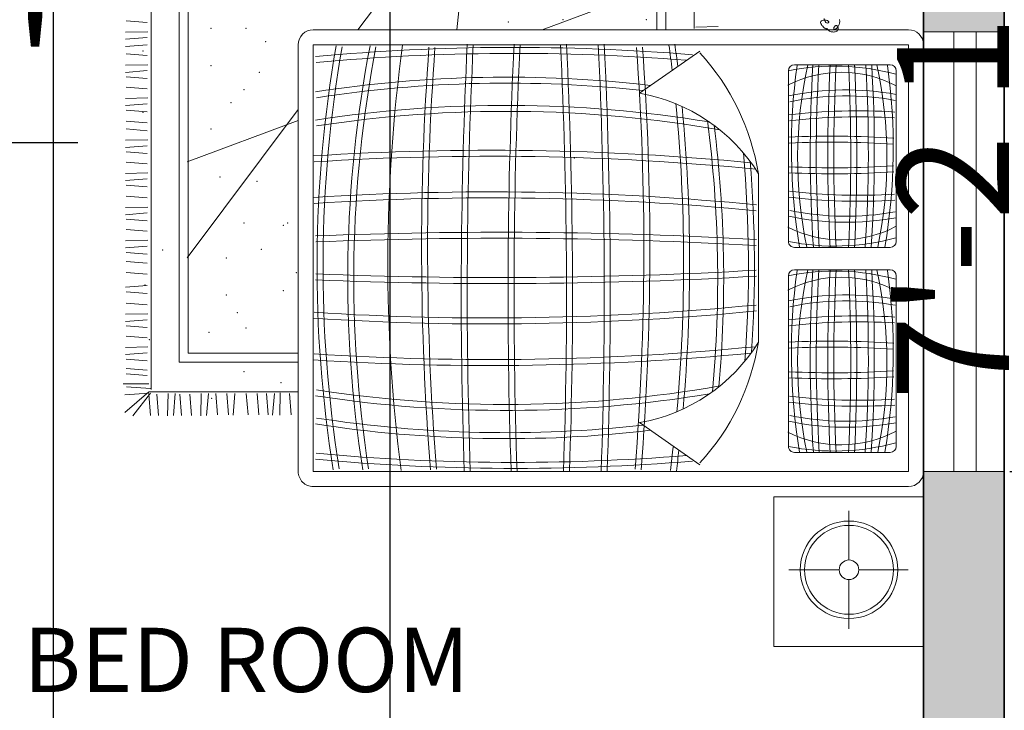
# Model space of a CAD drawing. Units: inches. Extents: x 1763 to 2368, y 1500 to 2097.
# Tile 14 of 24: x 2079 to 2189, y 1720 to 1797. Entities that reach past the tile are written whole.
import ezdxf

# ---------------------------------------------------------------- set-up
doc = ezdxf.new("R2010")
doc.units = ezdxf.units.IN
for name, color, linetype, lineweight in [('A-ANNO-DIMS', 2, 'Continuous', 18), ('A-AREA-IDEN', 7, 'Continuous', 18), ('A-FURN', 8, 'Continuous', 18), ('A-WALL', 7, 'Continuous', 35), ('A-WALL-PATT', 7, 'Continuous', 13), ('windows', 1, 'Continuous', 18)]:
    doc.layers.add(name, color=color, linetype=linetype, lineweight=lineweight)
doc.styles.get("Standard").update_dxf_attribs({"font": 'arial.ttf'})
doc.dimstyles.new('ISO-25', dxfattribs={"dimtxt": 12.5, "dimasz": 2.5, "dimexe": 1.25, "dimexo": 0.625, "dimtad": 1, "dimdec": 0, "dimlunit": 4, "dimtxsty": 'Standard', "dimblk": 'ARCHTICK', "dimcen": 2.5, "dimclrd": 3, "dimclrt": 4, "dimadec": 0, "dimazin": 0, "dimtfac": 1, "dimtdec": 0, "dimtmove": 0, "dimatfit": 3, "dimfxl": 1, "dimarcsym": 0})

# ---------------------------------------------------------------- blocks, each defined once
blk = doc.blocks.new('A$C77DF40FE')
for p, q in [((0.5839, 2.6714), (2.0097, 2.6714)), ((2.0936, 2.1723), (2.0936, 2.6723)), ((2.0936, 2.6723), (2.5936, 2.6723)), ((2.5936, 2.6723), (2.5936, 2.1723)), ((0.5339, 0.6344), (0.5339, 2.6214)), ((0.5839, 2.6214), (2.0097, 2.6214)), ((0.5839, 0.6344), (0.5839, 2.6214)), ((2.0097, 2.6214), (2.0097, 0.6344)), ((2.0597, 2.6214), (2.0597, 0.6344)), ((2.3379, 2.4554), (2.3379, 2.6199)), ((1.2408, 2.5803), (0.6708, 2.5803)), ((1.9255, 2.5803), (1.3555, 2.5803)), ((0.6508, 2.5603), (0.6508, 2.2403)), ((1.2608, 2.2403), (1.2608, 2.5603)), ((1.3355, 2.5603), (1.3355, 2.2403)), ((1.9455, 2.2403), (1.9455, 2.5603)), ((2.3051, 2.4226), (2.1406, 2.4226)), ((2.5352, 2.4226), (2.3707, 2.4226)), ((0.506, 2.3917), (0.5, 2.3914)), ((0.5117, 2.391), (0.506, 2.3917)), ((0.5168, 2.3897), (0.5117, 2.391)), ((0.5212, 2.3878), (0.5168, 2.3897)), ((0.5205, 2.3816), (0.5202, 2.3804)), ((0.5202, 2.3804), (0.5202, 2.379)), ((0.5202, 2.379), (0.5206, 2.3777)), ((0.521, 2.3828), (0.5205, 2.3816)), ((0.5206, 2.3777), (0.5213, 2.3764)), ((0.5219, 2.3839), (0.521, 2.3828)), ((0.5248, 2.3858), (0.5212, 2.3878)), ((0.5213, 2.3764), (0.5224, 2.3752)), ((0.523, 2.3849), (0.5219, 2.3839)), ((0.5224, 2.3752), (0.5237, 2.374)), ((0.5244, 2.3856), (0.523, 2.3849)), ((0.5237, 2.374), (0.5252, 2.3731)), ((0.5261, 2.3861), (0.5244, 2.3856)), ((0.5277, 2.3836), (0.5248, 2.3858)), ((0.5252, 2.3731), (0.5268, 2.3723)), ((0.5279, 2.3864), (0.5261, 2.3861)), ((0.5268, 2.3723), (0.5283, 2.3719)), ((0.5298, 2.3813), (0.5277, 2.3836)), ((0.5298, 2.3864), (0.5279, 2.3864)), ((0.5283, 2.3719), (0.5297, 2.3717)), ((0.5297, 2.3717), (0.531, 2.372)), ((0.5318, 2.3861), (0.5298, 2.3864)), ((0.5313, 2.3792), (0.5298, 2.3813)), ((0.531, 2.372), (0.5319, 2.3726)), ((0.5322, 2.3771), (0.5313, 2.3792)), ((0.5338, 2.3855), (0.5318, 2.3861)), ((0.5319, 2.3726), (0.5325, 2.3738)), ((0.5326, 2.3753), (0.5322, 2.3771)), ((0.5325, 2.3738), (0.5326, 2.3753)), ((0.5356, 2.3846), (0.5338, 2.3855)), ((0.5373, 2.3832), (0.5356, 2.3846)), ((0.5387, 2.3815), (0.5373, 2.3832)), ((0.5399, 2.3794), (0.5387, 2.3815)), ((0.5407, 2.377), (0.5399, 2.3794)), ((0.5412, 2.3743), (0.5407, 2.377)), ((0.5409, 2.3657), (0.5413, 2.3686)), ((0.5414, 2.3715), (0.5412, 2.3743)), ((0.5413, 2.3686), (0.5414, 2.3715)), ((2.3379, 2.2215), (2.3379, 2.3898)), ((0.4961, 2.3402), (0.5023, 2.3413)), ((0.502, 2.3463), (0.5017, 2.3431)), ((0.5017, 2.3431), (0.5018, 2.3398)), ((0.5018, 2.3398), (0.5023, 2.3365)), ((0.5026, 2.3491), (0.502, 2.3463)), ((0.5023, 2.3413), (0.5067, 2.3431)), ((0.5023, 2.3365), (0.5031, 2.3334)), ((0.5035, 2.3514), (0.5026, 2.3491)), ((0.5031, 2.3334), (0.5043, 2.3309)), ((0.5047, 2.3531), (0.5035, 2.3514)), ((0.5059, 2.3542), (0.5047, 2.3531)), ((0.5073, 2.3548), (0.5059, 2.3542)), ((0.5067, 2.3431), (0.5095, 2.3452)), ((0.5086, 2.3549), (0.5073, 2.3548)), ((0.5097, 2.3544), (0.5086, 2.3549)), ((0.5095, 2.3452), (0.511, 2.3475)), ((0.5107, 2.3534), (0.5097, 2.3544)), ((0.5113, 2.3518), (0.5107, 2.3534)), ((0.511, 2.3475), (0.5115, 2.3498)), ((0.5115, 2.3498), (0.5113, 2.3518)), ((0.5193, 2.3325), (0.5222, 2.3349)), ((0.5222, 2.3349), (0.5249, 2.3374)), ((0.5249, 2.3374), (0.5271, 2.3398)), ((0.5271, 2.3398), (0.5288, 2.3419)), ((0.5288, 2.3419), (0.5299, 2.3436)), ((0.5299, 2.3436), (0.5305, 2.3449)), ((0.53, 2.3482), (0.5302, 2.3488)), ((0.5301, 2.3477), (0.53, 2.3482)), ((0.5303, 2.3472), (0.5301, 2.3477)), ((0.5302, 2.3488), (0.5308, 2.3495)), ((0.5306, 2.3466), (0.5303, 2.3472)), ((0.5305, 2.3449), (0.5307, 2.3459)), ((0.5307, 2.3459), (0.5306, 2.3466)), ((0.5308, 2.3495), (0.5317, 2.3504)), ((0.5317, 2.3504), (0.5329, 2.3515)), ((0.5329, 2.3515), (0.5342, 2.3528)), ((0.5342, 2.3528), (0.5356, 2.3543)), ((0.5356, 2.3543), (0.537, 2.3561)), ((0.537, 2.3561), (0.5383, 2.3581)), ((0.5383, 2.3581), (0.5394, 2.3604)), ((0.5394, 2.3604), (0.5403, 2.3629)), ((0.5403, 2.3629), (0.5409, 2.3657)), ((0.5043, 2.3309), (0.506, 2.329)), ((0.506, 2.329), (0.5081, 2.328)), ((0.5081, 2.328), (0.5106, 2.328)), ((0.5106, 2.328), (0.5134, 2.3288)), ((0.5134, 2.3288), (0.5163, 2.3304)), ((0.5163, 2.3304), (0.5193, 2.3325)), ((0.6708, 2.2203), (1.2408, 2.2203)), ((1.3555, 2.2203), (1.9255, 2.2203)), ((2.5936, 2.1723), (2.0936, 2.1723)), ((1.5773, 2.1205), (1.0147, 2.1205)), ((0.5249, 1.9118), (0.5233, 1.9865)), ((0.6051, 1.925), (0.7457, 1.7234)), ((1.9869, 1.925), (1.8463, 1.7234)), ((0.5301, 1.9057), (0.3112, 1.9057)), ((0.5339, 1.8116), (0.3112, 1.8116)), ((0.5339, 1.7816), (0.3112, 1.7816)), ((0.3909, 1.7821), (0.5339, 1.398)), ((0.5339, 1.1132), (0.2152, 1.1479)), ((0.5339, 0.7837), (0.2152, 1.0221)), ((2.0097, 0.6344), (0.5839, 0.6344)), ((2.0097, 0.5844), (0.5839, 0.5844)), ((1.2963, 0.2134), (0.8003, 0.5844)), ((0.8369, 0.5844), (0.975, 0.2134)), ((1.6139, 0.217), (1.6139, 0.5844)), ((1.6439, 0.187), (1.6439, 0.5844)), ((1.7439, 0.087), (1.7439, 0.5844)), ((1.8197, 0.5605), (1.7489, 0.5548)), ((1.8218, 0.5229), (1.7471, 0.5245)), ((1.8218, 0.499), (1.7487, 0.5048)), ((1.8197, 0.4839), (1.7489, 0.4783)), ((1.8197, 0.453), (1.7489, 0.4474)), ((1.8197, 0.4168), (1.7489, 0.4111)), ((1.8218, 0.3671), (1.7487, 0.3728)), ((1.8197, 0.352), (1.7489, 0.3463)), ((1.8197, 0.3146), (1.7489, 0.3089)), ((1.7492, 0.2844), (1.8223, 0.2787)), ((1.7492, 0.2606), (1.824, 0.2589)), ((0.3112, 0.217), (1.6139, 0.217)), ((1.7513, 0.223), (1.8221, 0.2286)), ((0.3112, 0.187), (1.6439, 0.187)), ((1.7492, 0.1737), (1.8223, 0.1679)), ((1.7513, 0.1888), (1.8221, 0.1944)), ((1.7492, 0.1499), (1.824, 0.1482)), ((1.7513, 0.1122), (1.8221, 0.1179)), ((0.3112, 0.0935), (1.0155, 0.0935)), ((0.5043, 0.0096), (0.51, 0.0804)), ((0.542, 0.0075), (0.5403, 0.0823)), ((0.5658, 0.0075), (0.56, 0.0806)), ((0.5896, 0.0075), (0.5838, 0.0806)), ((0.6147, 0.0096), (0.6204, 0.0804)), ((0.6523, 0.0075), (0.6507, 0.0823)), ((0.6762, 0.0075), (0.6704, 0.0806)), ((0.6912, 0.0096), (0.6969, 0.0804)), ((0.7254, 0.0096), (0.7311, 0.0804)), ((0.7631, 0.0075), (0.7614, 0.0823)), ((0.7869, 0.0075), (0.7811, 0.0806)), ((0.802, 0.0096), (0.8076, 0.0804)), ((0.8394, 0.0096), (0.8451, 0.0804)), ((0.8654, 0.0096), (0.8711, 0.0804)), ((0.9031, 0.0075), (0.9014, 0.0823)), ((0.9269, 0.0075), (0.9212, 0.0806)), ((0.942, 0.0096), (0.9477, 0.0804)), ((0.9762, 0.0096), (0.9818, 0.0804)), ((1.0138, 0.0075), (1.0122, 0.0823)), ((1.0155, 0.0935), (1.7355, 0.0935)), ((1.0376, 0.0075), (1.0319, 0.0806)), ((1.0527, 0.0096), (1.0584, 0.0804)), ((1.0901, 0.0096), (1.0958, 0.0804)), ((1.1278, 0.0075), (1.1261, 0.0823)), ((1.1516, 0.0075), (1.1459, 0.0806)), ((1.1667, 0.0096), (1.1724, 0.0804)), ((1.2009, 0.0096), (1.2065, 0.0804)), ((1.2385, 0.0075), (1.2368, 0.0823)), ((1.2623, 0.0075), (1.2566, 0.0806)), ((1.2774, 0.0096), (1.2831, 0.0804)), ((1.3083, 0.0096), (1.314, 0.0804)), ((1.3446, 0.0096), (1.3503, 0.0804)), ((1.3943, 0.0075), (1.3885, 0.0806)), ((1.4094, 0.0096), (1.415, 0.0804)), ((1.4468, 0.0096), (1.4525, 0.0804)), ((1.4844, 0.0075), (1.4828, 0.0823)), ((1.5083, 0.0075), (1.5025, 0.0806)), ((1.5233, 0.0096), (1.529, 0.0804)), ((1.5575, 0.0096), (1.5632, 0.0804)), ((1.5951, 0.0075), (1.5935, 0.0823)), ((1.619, 0.0075), (1.6132, 0.0806)), ((1.6341, 0.0096), (1.6397, 0.0804)), ((1.665, 0.0096), (1.6706, 0.0804)), ((1.6831, 0.0096), (1.6888, 0.0804)), ((1.7162, 0.0857), (1.7162, 0)), ((1.7323, 0.0911), (1.7269, 0.0107)), ((1.743, 0.0857), (1.8126, 0.0054)), ((1.7483, 0.0911), (1.8233, 0.0322)), ((1.7483, 0.0857), (1.7537, 0.0054)), ((1.7513, 0.0858), (1.8221, 0.0915))]:
    blk.add_line(p, q)
for radius in [0.1629, 0.1484, 0.0328]:
    blk.add_circle((2.3379, 2.4226), radius)
for centre, radius, start, end in [((0.5839, 2.6214), 0.05, 90, 180), ((2.0097, 2.6214), 0.05, 0, 90), ((0.6708, 2.5603), 0.02, 90, 180), ((0.9287, 0.5819), 1.9884, 80.4201, 97.9672), ((1.4247, 2.3742), 0.7696, 164.6112, 191.5679), ((1.0701, 2.3966), 0.3942, 152.5365, 206.92), ((1.6628, 2.4129), 0.928, 169.6087, 191.899), ((1.6628, 2.4129), 0.908, 169.6087, 191.899), ((2.7571, 2.4533), 1.9523, 176.3947, 186.8195), ((2.7571, 2.4533), 1.9323, 176.3947, 186.8195), ((3.9259, 2.3685), 3.0367, 176.1432, 182.775), ((3.9259, 2.3685), 3.0167, 176.1432, 182.775), ((-2.0216, 2.3685), 3.0167, 357.225, 3.8568), ((-2.0216, 2.3685), 3.0367, 357.225, 3.8568), ((-0.8455, 2.4533), 1.9323, 353.1805, 3.6053), ((-0.8455, 2.4533), 1.9523, 353.1805, 3.6053), ((0.2489, 2.4129), 0.908, 348.101, 10.3913), ((0.2489, 2.4129), 0.928, 348.101, 10.3913), ((0.8416, 2.3966), 0.3942, 333.08, 27.4635), ((0.4869, 2.3742), 0.7696, 348.4321, 15.3888), ((1.2408, 2.5603), 0.02, 0, 90), ((1.3555, 2.5603), 0.02, 90, 180), ((1.6135, 0.5819), 1.9884, 80.4201, 97.9672), ((2.1094, 2.3742), 0.7696, 164.6112, 191.5679), ((1.7548, 2.3966), 0.3942, 152.5365, 206.92), ((2.3475, 2.4129), 0.928, 169.6087, 191.899), ((2.3475, 2.4129), 0.908, 169.6087, 191.899), ((3.4419, 2.4533), 1.9523, 176.3947, 186.8195), ((3.4419, 2.4533), 1.9323, 176.3947, 186.8195), ((4.6106, 2.3685), 3.0367, 176.1432, 182.775), ((4.6106, 2.3685), 3.0167, 176.1432, 182.775), ((-1.3369, 2.3685), 3.0167, 357.225, 3.8568), ((-1.3369, 2.3685), 3.0367, 357.225, 3.8568), ((-0.1608, 2.4533), 1.9323, 353.1805, 3.6053), ((-0.1608, 2.4533), 1.9523, 353.1805, 3.6053), ((0.9336, 2.4129), 0.908, 348.101, 10.3913), ((0.9336, 2.4129), 0.928, 348.101, 10.3913), ((1.5263, 2.3966), 0.3942, 333.08, 27.4635), ((1.1716, 2.3742), 0.7696, 348.4321, 15.3888), ((1.9255, 2.5603), 0.02, 0, 90), ((0.9635, 1.1066), 1.4427, 78.1527, 102.4906), ((1.6482, 1.1066), 1.4427, 78.1527, 102.4906), ((0.9445, -2.3575), 4.8647, 86.2671, 93.4563), ((1.6292, -2.3575), 4.8647, 86.2671, 93.4563), ((0.9445, -2.3575), 4.8447, 86.2671, 93.4563), ((1.6292, -2.3575), 4.8447, 86.2671, 93.4563), ((0.9561, -3.928), 6.3765, 87.24779, 92.75221), ((1.6408, -3.928), 6.3765, 87.24779, 92.75221), ((0.9561, -3.928), 6.3565, 87.24779, 92.75221), ((1.6408, -3.928), 6.3565, 87.24779, 92.75221), ((0.9561, 8.7285), 6.3565, 267.24779, 272.75221), ((1.6408, 8.7285), 6.3565, 267.24779, 272.75221), ((0.9561, 8.7285), 6.3765, 267.24779, 272.75221), ((1.6408, 8.7285), 6.3765, 267.24779, 272.75221), ((0.9445, 7.158), 4.8647, 266.5437, 273.7329), ((0.9445, 7.158), 4.8447, 266.5437, 273.7329), ((1.6292, 7.158), 4.8647, 266.5437, 273.7329), ((1.6292, 7.158), 4.8447, 266.5437, 273.7329), ((0.9635, 3.6939), 1.4427, 257.5094, 281.8473), ((1.6482, 3.6939), 1.4427, 257.5094, 281.8473), ((0.6708, 2.2403), 0.02, 180, 270), ((0.9287, 4.2186), 1.9884, 262.0328, 279.5799), ((1.2408, 2.2403), 0.02, 270, 0), ((1.3555, 2.2403), 0.02, 180, 270), ((1.6135, 4.2186), 1.9884, 262.0328, 279.5799), ((1.9255, 2.2403), 0.02, 270, 0), ((1.1396, 1.3485), 0.782, 99.1908, 132.5116), ((1.3217, 1.6229), 0.5847, 121.6676, 170.1065), ((10.1174, 1.2237), 9.161, 174.43278, 183.67204), ((1.3248, -2.1722), 4.2793, 86.1532, 94.7091), ((10.2564, 1.2237), 9.181, 174.43278, 183.67204), ((10.2564, 1.2237), 9.161, 174.43278, 183.67204), ((16.3019, 1.253), 15.0916, 176.72768, 182.32074), ((16.3019, 1.253), 15.0716, 176.72768, 182.32074), ((-13.7099, 1.253), 15.0716, 357.67926, 3.27232), ((-13.7099, 1.253), 15.0916, 357.67926, 3.27232), ((-7.6644, 1.2237), 9.161, 356.32796, 5.56722), ((-7.6644, 1.2237), 9.181, 356.32796, 5.56722), ((1.2703, 1.6229), 0.5847, 9.8935, 58.3324), ((1.4523, 1.3485), 0.782, 47.4884, 80.8092), ((-7.5254, 1.2237), 9.161, 356.32796, 5.55658), ((10.1174, 1.2237), 9.181, 174.54912, 183.67204), ((1.3248, -2.1722), 4.2593, 85.7473, 95.1159), ((-7.5254, 1.2237), 9.181, 356.32796, 5.45088), ((4.947, 1.2796), 4.1406, 170.0939, 188.8179), ((1.3657, -2.1044), 4.0888, 84.7053, 97.4283), ((1.3657, -2.1044), 4.1088, 84.9619, 97.1707), ((-2.355, 1.2796), 4.1406, 351.1821, 9.9061), ((4.947, 1.2796), 4.1606, 170.6272, 188.8179), ((-2.355, 1.2796), 4.1606, 351.1821, 9.3728), ((7.8077, 1.3061), 7.2149, 175.27403, 185.28261), ((7.8077, 1.3061), 7.1949, 175.41729, 185.28261), ((1.3142, -3.5764), 5.4671, 84.8953, 95.5052), ((-5.2157, 1.3061), 7.1949, 354.71739, 4.58271), ((-5.2157, 1.3061), 7.2149, 354.71739, 4.72597), ((1.3142, -3.5764), 5.4671, 96.9078, 97.6924), ((1.3142, -3.5764), 5.4471, 84.7792, 95.6214), ((1.3142, -3.5764), 5.4671, 82.7025, 83.4474), ((1.3142, -3.5764), 5.4471, 96.796, 97.6924), ((1.3142, -3.5764), 5.4471, 82.7025, 83.5609), ((1.2659, -7.4764), 9.2344, 85.41732, 94.18368), ((4.8527, 1.2796), 4.1606, 173.3677, 188.8179), ((-2.2608, 1.2796), 4.1606, 351.1821, 6.6323), ((1.2659, -7.4764), 9.2144, 85.41732, 94.18368), ((4.8527, 1.2796), 4.1406, 173.6812, 188.8179), ((-2.2608, 1.2796), 4.1406, 351.1821, 6.3188), ((1.4138, -15.5462), 17.172, 88.01473, 92.775), ((1.4138, -15.5462), 17.152, 88.01473, 92.775), ((1.4138, -15.6721), 17.172, 88.01473, 92.775), ((1.4138, -15.6721), 17.152, 88.01473, 92.775), ((1.4138, 18.4566), 17.152, 267.225, 271.98527), ((1.4138, 18.4566), 17.172, 267.225, 271.98527), ((1.4138, 18.3004), 17.152, 267.225, 271.98527), ((1.4138, 18.3004), 17.172, 267.225, 271.98527), ((1.2659, 10.2305), 9.2344, 265.81632, 274.58268), ((1.2659, 10.2305), 9.2144, 265.81632, 274.58268), ((1.3142, 6.3306), 5.4471, 262.3076, 277.2975), ((1.3657, 4.8586), 4.1088, 259.0794, 278.9327), ((1.3657, 4.8586), 4.0888, 259.0794, 278.9327), ((1.3248, 4.9264), 4.2593, 260.0761, 279.1287), ((1.3248, 4.9264), 4.2793, 260.0761, 279.1287), ((0.5839, 0.6344), 0.05, 180, 270), ((2.0097, 0.6344), 0.05, 270, 0)]:
    blk.add_arc(centre, radius, start, end)
for p in [(0.5004, 1.7457), (0.9622, 1.5058), (0.5004, 1.4684), (0.5077, 1.286), (1.3453, 0.5782), (1.1794, 0.5491), (1.1867, 0.5345), (1.4058, 0.5345), (1.7124, 0.5272), (0.5734, 0.4761), (1.2671, 0.4615), (0.6757, 0.4542), (1.0407, 0.4469), (0.5296, 0.4104), (0.7341, 0.4032), (1.1794, 0.4032), (1.5299, 0.4104), (1.6759, 0.4032), (1.4788, 0.3813), (0.7779, 0.3594), (1.2963, 0.3448), (1.4204, 0.3448), (1.0261, 0.3229), (0.5296, 0.2937), (0.6538, 0.2937), (0.8655, 0.2937), (1.5445, 0.2864), (1.7652, 0.2958), (1.2693, 0.1315), (0.6049, 0.0659), (0.8093, 0.0659), (1.3861, 0.0732), (1.5686, 0.0878)]:
    blk.add_point(p)
blk = doc.blocks.new('_ArchTick')
at = {"color": 0, "linetype": 'ByBlock', "const_width": 0.15}
blk.add_lwpolyline([(-0.5, -0.5), (0.5, 0.5)], dxfattribs=at)
blk = doc.blocks.new('*D22')
at = {"layer": 'A-ANNO-DIMS', "color": 0, "lineweight": -2, "transparency": 16777216}
for p, q in [((2189.72, 2043.27), (2269.32, 2043.27)), ((2268.07, 2043.27), (2268.07, 1563.27)), ((2189.72, 1563.27), (2269.32, 1563.27))]:
    blk.add_line(p, q, dxfattribs=at)
at = {"layer": 'Defpoints', "color": 0, "transparency": 16777216}
for p in [(2189.09, 2043.27), (2189.09, 1563.27), (2268.07, 1563.27)]:
    blk.add_point(p, dxfattribs=at)
at = {"layer": 'A-ANNO-DIMS', "color": 0, "lineweight": -2, "transparency": 16777216, "xscale": 2.5, "yscale": 2.5, "zscale": 2.5}
for p, rotation in [((2268.07, 2043.27), 90), ((2268.07, 1563.27), 270)]:
    blk.add_blockref('_ArchTick', p, dxfattribs=dict(at, rotation=rotation))
at = {"layer": 'A-ANNO-DIMS', "color": 0, "transparency": 16777216, "insert": (2261.06, 1803.27), "char_height": 12.5, "attachment_point": 5, "rotation": 90}
blk.add_mtext("40'", dxfattribs=at)
blk = doc.blocks.new('*D24')
at = {"layer": 'A-ANNO-DIMS', "color": 0, "lineweight": -2, "transparency": 16777216}
for p, q in [((2179.32, 1949.35), (2193.33, 1949.35)), ((2179.32, 1862.76), (2193.33, 1862.76))]:
    blk.add_line(p, q, dxfattribs=at)
at = {"layer": 'A-ANNO-DIMS', "color": 3, "lineweight": -2, "transparency": 16777216}
for p, q in [((2192.08, 1949.35), (2192.08, 1862.76)), ((2192.08, 1862.76), (2192.08, 1753.79))]:
    blk.add_line(p, q, dxfattribs=at)
at = {"layer": 'Defpoints', "color": 0, "transparency": 16777216}
for p in [(2178.7, 1949.35), (2178.7, 1862.76), (2192.08, 1862.76)]:
    blk.add_point(p, dxfattribs=at)
at = {"layer": 'A-ANNO-DIMS', "color": 3, "lineweight": -2, "transparency": 16777216, "xscale": 2.5, "yscale": 2.5, "zscale": 2.5}
for p, rotation in [((2192.08, 1949.35), 90), ((2192.08, 1862.76), 270)]:
    blk.add_blockref('_ArchTick', p, dxfattribs=dict(at, rotation=rotation))
at = {"layer": 'A-ANNO-DIMS', "color": 4, "transparency": 16777216, "insert": (2184.99, 1807.02), "char_height": 12.5, "attachment_point": 5, "rotation": 90}
blk.add_mtext('7\'-2 1/2" TYP.', dxfattribs=at)
blk = doc.blocks.new('*D27')
at = {"layer": 'A-ANNO-DIMS', "color": 0, "lineweight": -2, "transparency": 16777216}
for p, q in [((1853.71, 1795.96), (1853.71, 1781.68)), ((1944.71, 1795.96), (1944.71, 1781.68))]:
    blk.add_line(p, q, dxfattribs=at)
at = {"layer": 'A-ANNO-DIMS', "color": 3, "lineweight": -2, "transparency": 16777216}
for p, q in [((1853.71, 1782.93), (1944.71, 1782.93)), ((1944.71, 1782.93), (2085.85, 1782.93))]:
    blk.add_line(p, q, dxfattribs=at)
at = {"layer": 'Defpoints', "color": 0, "transparency": 16777216}
for p in [(1853.71, 1796.58), (1944.71, 1796.58), (1944.71, 1782.93)]:
    blk.add_point(p, dxfattribs=at)
at = {"layer": 'A-ANNO-DIMS', "color": 3, "lineweight": -2, "transparency": 16777216, "xscale": 2.5, "yscale": 2.5, "zscale": 2.5, "rotation": 180}
blk.add_blockref('_ArchTick', (1853.71, 1782.93), dxfattribs=at)
at = {"layer": 'A-ANNO-DIMS', "color": 3, "lineweight": -2, "transparency": 16777216, "xscale": 2.5, "yscale": 2.5, "zscale": 2.5}
blk.add_blockref('_ArchTick', (1944.71, 1782.93), dxfattribs=at)
at = {"layer": 'A-ANNO-DIMS', "color": 4, "transparency": 16777216, "insert": (2016.53, 1790.02), "char_height": 12.5, "attachment_point": 5}
blk.add_mtext('DINING SET 7\'-7"', dxfattribs=at)
blk = doc.blocks.new('*D52')
at = {"layer": 'A-ANNO-DIMS', "color": 0, "lineweight": -2, "transparency": 16777216}
for p, q in [((2189.72, 1746.22), (2217.84, 1746.22)), ((2180.72, 1679.27), (2217.84, 1679.27))]:
    blk.add_line(p, q, dxfattribs=at)
at = {"layer": 'A-ANNO-DIMS', "color": 3, "lineweight": -2, "transparency": 16777216}
blk.add_line((2216.59, 1679.27), (2216.59, 1746.22), dxfattribs=at)
at = {"layer": 'Defpoints', "color": 0, "transparency": 16777216}
for p in [(2189.09, 1746.22), (2216.59, 1746.22), (2180.09, 1679.27)]:
    blk.add_point(p, dxfattribs=at)
at = {"layer": 'A-ANNO-DIMS', "color": 3, "lineweight": -2, "transparency": 16777216, "xscale": 2.5, "yscale": 2.5, "zscale": 2.5}
for p, rotation in [((2216.59, 1746.22), 90), ((2216.59, 1679.27), 270)]:
    blk.add_blockref('_ArchTick', p, dxfattribs=dict(at, rotation=rotation))
at = {"layer": 'A-ANNO-DIMS', "color": 4, "transparency": 16777216, "insert": (2209.61, 1712.75), "char_height": 12.5, "attachment_point": 5, "rotation": 90}
blk.add_mtext('5\'-7"', dxfattribs=at)
blk = doc.blocks.new('*D62')
at = {"layer": 'A-ANNO-DIMS', "color": 0, "lineweight": -2, "transparency": 16777216}
for p, q in [((2083.09, 1980.65), (2083.09, 1509.91)), ((2120.61, 1980.65), (2120.61, 1509.91))]:
    blk.add_line(p, q, dxfattribs=at)
at = {"layer": 'A-ANNO-DIMS', "color": 3, "lineweight": -2, "transparency": 16777216}
for p, q in [((2083.09, 1511.16), (2120.61, 1511.16)), ((2120.61, 1511.16), (2186.71, 1511.16))]:
    blk.add_line(p, q, dxfattribs=at)
at = {"layer": 'Defpoints', "color": 0, "transparency": 16777216}
for p in [(2083.09, 1981.27), (2120.61, 1981.27), (2120.61, 1511.16)]:
    blk.add_point(p, dxfattribs=at)
at = {"layer": 'A-ANNO-DIMS', "color": 3, "lineweight": -2, "transparency": 16777216, "xscale": 2.5, "yscale": 2.5, "zscale": 2.5, "rotation": 180}
blk.add_blockref('_ArchTick', (2083.09, 1511.16), dxfattribs=at)
at = {"layer": 'A-ANNO-DIMS', "color": 3, "lineweight": -2, "transparency": 16777216, "xscale": 2.5, "yscale": 2.5, "zscale": 2.5}
blk.add_blockref('_ArchTick', (2120.61, 1511.16), dxfattribs=at)
at = {"layer": 'A-ANNO-DIMS', "color": 4, "transparency": 16777216, "insert": (2154.91, 1518.25), "char_height": 12.5, "attachment_point": 5}
blk.add_mtext('3\'-1 1/2"', dxfattribs=at)
blk = doc.blocks.new('*D71')
at = {"layer": 'A-ANNO-DIMS', "color": 0, "lineweight": -2, "transparency": 16777216}
for p, q in [((2049.69, 1879.65), (2049.69, 1509.91)), ((2072.78, 1879.65), (2072.78, 1509.91))]:
    blk.add_line(p, q, dxfattribs=at)
at = {"layer": 'A-ANNO-DIMS', "color": 3, "lineweight": -2, "transparency": 16777216}
for p, q in [((2049.69, 1511.16), (2072.78, 1511.16)), ((2072.78, 1511.16), (2118.3, 1511.16))]:
    blk.add_line(p, q, dxfattribs=at)
at = {"layer": 'Defpoints', "color": 0, "transparency": 16777216}
for p in [(2049.69, 1880.27), (2072.78, 1880.27), (2072.78, 1511.16)]:
    blk.add_point(p, dxfattribs=at)
at = {"layer": 'A-ANNO-DIMS', "color": 3, "lineweight": -2, "transparency": 16777216, "xscale": 2.5, "yscale": 2.5, "zscale": 2.5, "rotation": 180}
blk.add_blockref('_ArchTick', (2049.69, 1511.16), dxfattribs=at)
at = {"layer": 'A-ANNO-DIMS', "color": 3, "lineweight": -2, "transparency": 16777216, "xscale": 2.5, "yscale": 2.5, "zscale": 2.5}
blk.add_blockref('_ArchTick', (2072.78, 1511.16), dxfattribs=at)
at = {"layer": 'A-ANNO-DIMS', "color": 4, "transparency": 16777216, "insert": (2096.79, 1518.06), "char_height": 12.5, "attachment_point": 5}
blk.add_mtext('1\'-11"', dxfattribs=at)

msp = doc.modelspace()

# ---------------------------------------------------------------- hatches: boundary and pattern name
at = {"layer": 'A-WALL-PATT'}
h = msp.add_hatch(color=256, dxfattribs=at)
h.dxf.hatch_style = 1
h.paths.add_polyline_path([(1838.09, 2034.27), (1838.09, 2043.27), (1829.09, 2043.27), (1829.09, 1953.39), (1838.09, 1953.39)])
h.paths.add_polyline_path([(1838.09, 1913.1), (1829.09, 1913.1), (1829.09, 1862.2), (1838.09, 1862.2)])
h.paths.add_polyline_path([(1838.09, 1825.59), (1829.09, 1825.59), (1829.09, 1738.64), (1838.09, 1738.64)])
h.paths.add_polyline_path([(1895.59, 1885.27), (1838.09, 1885.27), (1838.09, 1880.27), (1895.59, 1880.27)])
h.paths.add_polyline_path([(1857.39, 1784.27), (1838.09, 1784.27), (1838.09, 1779.27), (1857.39, 1779.27)])
h.paths.add_polyline_path([(1958.09, 1981.27), (1971.46, 1981.27), (1971.46, 1986.27), (1968.57, 1986.27), (1958.09, 1986.27), (1953.09, 1986.27), (1927.39, 1986.27), (1927.39, 1981.27), (1953.09, 1981.27), (1953.09, 1885.27), (1932.01, 1885.27), (1932.01, 1880.27), (1959.13, 1880.27), (1959.13, 1883.74), (1959.13, 1885.27), (1958.09, 1885.27)])
h.paths.add_polyline_path([(2018.09, 1981.27), (2031.02, 1981.27), (2031.02, 1986.27), (2018.09, 1986.27), (2013.09, 1986.27), (2001.23, 1986.27), (2001.23, 1981.27), (2013.09, 1981.27), (2013.09, 1885.27), (1982.18, 1885.27, -0.016629), (1982.23, 1883.74), (1982.23, 1880.27), (2049.69, 1880.27), (2049.69, 1883.74, -0.016629), (2049.74, 1885.27), (2018.09, 1885.27)])
h.paths.add_polyline_path([(2083.09, 1981.27), (2120.61, 1981.27), (2120.61, 1986.27), (2083.09, 1986.27), (2078.09, 1986.27), (2063.14, 1986.27), (2063.14, 1981.27), (2078.09, 1981.27), (2078.09, 1885.27), (2072.78, 1885.27), (2072.78, 1883.74), (2072.78, 1880.27), (2078.09, 1880.27), (2078.09, 1866.87), (2081.56, 1866.87, -0.016629), (2083.09, 1866.82)])
h.paths.add_polyline_path([(1871.68, 1635.27), (1838.09, 1635.27), (1838.09, 1626.27), (1871.68, 1626.27)], flags=17)
h.paths.add_polyline_path([(2100.58, 1688.27), (2060.09, 1688.27), (2060.09, 1679.27), (2100.58, 1679.27)], flags=17)
h.paths.add_polyline_path([(2180.09, 1688.27), (2148.74, 1688.27), (2148.74, 1679.27), (2180.09, 1679.27)], flags=17)
h.paths.add_polyline_path([(2189.09, 1746.22), (2180.09, 1746.22), (2180.09, 1743.42), (2180.12, 1743.42), (2180.12, 1726.72), (2180.09, 1572.27), (2034.91, 1572.27), (2034.91, 1565.6), (2034.91, 1563.27), (2189.09, 1563.27)])
h.paths.add_polyline_path([(2060.09, 1802.35, -0.016629), (2058.56, 1802.3), (2055.09, 1802.3), (2055.09, 1635.27), (2042.48, 1635.27), (2042.48, 1629.74), (2042.48, 1626.27), (2055.09, 1626.27), (2055.09, 1599.27), (2040.27, 1599.27), (2040.27, 1590.27), (2060.09, 1590.27)])
h.paths.add_polyline_path([(2019.39, 1629.74, -0.060569), (2020.06, 1635.27), (1995.09, 1635.27), (1990.09, 1635.27), (1927.07, 1635.27), (1927.07, 1626.27), (1990.09, 1626.27), (1990.09, 1590.27), (1995.09, 1590.27), (2005.2, 1590.27), (2005.2, 1599.27), (1995.09, 1599.27), (1995.09, 1626.27), (2019.39, 1626.27)])
edge = h.paths.add_edge_path()
edge.add_line((2180.09, 1837.27), (2167.2, 1837.27))
edge.add_spline(control_points=[(2167.2, 1837.27), (2167.19, 1837.27), (2167.18, 1837.27), (2167.18, 1837.27)], knot_values=[168.955493, 168.955493, 168.955493, 168.955493, 169.065871, 169.065871, 169.065871, 169.065871], degree=3, periodic=0)
edge.add_spline(control_points=[(2167.18, 1837.27), (2166.56, 1837.38), (2166.33, 1846.16), (2165.71, 1846.24)], knot_values=[159.864705, 159.864705, 159.864705, 159.864705, 168.955493, 168.955493, 168.955493, 168.955493], degree=3, periodic=0)
edge.add_line((2167.12, 1837.27), (2163.16, 1837.27))
edge.add_spline(control_points=[(2163.16, 1837.27), (2163.16, 1837.27), (2163.16, 1837.27), (2163.15, 1837.27)], knot_values=[150.537172, 150.537172, 150.537172, 150.537172, 150.553797, 150.553797, 150.553797, 150.553797], degree=3, periodic=0)
edge.add_spline(control_points=[(2163.15, 1837.27), (2162.29, 1837.29), (2161.59, 1846.23), (2160.88, 1846.24)], knot_values=[141.293426, 141.293426, 141.293426, 141.293426, 150.537172, 150.537172, 150.537172, 150.537172], degree=3, periodic=0)
edge.add_line((2163.08, 1837.27), (2158.7, 1837.27))
edge.add_spline(control_points=[(2158.7, 1837.27), (2158.7, 1837.27), (2158.7, 1837.27), (2158.7, 1837.27)], knot_values=[132.033544, 132.033544, 132.033544, 132.033544, 132.049151, 132.049151, 132.049151, 132.049151], degree=3, periodic=0)
edge.add_spline(control_points=[(2158.7, 1837.27), (2157.97, 1837.29), (2157.26, 1846.23), (2156.39, 1846.24)], knot_values=[122.786021, 122.786021, 122.786021, 122.786021, 132.033544, 132.033544, 132.033544, 132.033544], degree=3, periodic=0)
edge.add_line((2158.63, 1837.27), (2153.84, 1837.27))
edge.add_spline(control_points=[(2153.84, 1837.27), (2153.83, 1837.27), (2153.82, 1837.27), (2153.82, 1837.27)], knot_values=[113.451585, 113.451585, 113.451585, 113.451585, 113.562103, 113.562103, 113.562103, 113.562103], degree=3, periodic=0)
edge.add_spline(control_points=[(2153.82, 1837.27), (2153.17, 1837.38), (2152.88, 1846.19), (2152.4, 1846.24)], knot_values=[0, 0, 0, 0, 9.081854, 9.081854, 9.081854, 9.081854], degree=3, periodic=0)
edge.add_line((2153.76, 1837.27), (2150.39, 1837.27))
edge.add_spline(control_points=[(2150.39, 1837.27), (2150.38, 1837.27), (2150.37, 1837.27), (2150.36, 1837.27)], knot_values=[95.069382, 95.069382, 95.069382, 95.069382, 95.17519, 95.17519, 95.17519, 95.17519], degree=3, periodic=0)
edge.add_spline(control_points=[(2150.36, 1837.27), (2149.49, 1837.37), (2148.42, 1846.19), (2147.59, 1846.24)], knot_values=[85.824599, 85.824599, 85.824599, 85.824599, 95.069382, 95.069382, 95.069382, 95.069382], degree=3, periodic=0)
edge.add_line((2150.29, 1837.27), (2145.43, 1837.27))
edge.add_spline(control_points=[(2145.43, 1837.27), (2145.43, 1837.27), (2145.42, 1837.27), (2145.42, 1837.27)], knot_values=[76.505559, 76.505559, 76.505559, 76.505559, 76.547811, 76.547811, 76.547811, 76.547811], degree=3, periodic=0)
edge.add_spline(control_points=[(2145.42, 1837.27), (2144.68, 1837.31), (2143.8, 1846.19), (2142.95, 1846.24)], knot_values=[67.23945, 67.23945, 67.23945, 67.23945, 76.505559, 76.505559, 76.505559, 76.505559], degree=3, periodic=0)
edge.add_line((2145.35, 1837.27), (2134.57, 1837.27))
edge.add_spline(control_points=[(2134.57, 1837.27), (2134.57, 1837.27), (2134.56, 1837.27), (2134.56, 1837.27)], knot_values=[39.001463, 39.001463, 39.001463, 39.001463, 39.045107, 39.045107, 39.045107, 39.045107], degree=3, periodic=0)
edge.add_spline(control_points=[(2134.56, 1837.27), (2133.87, 1837.31), (2133.4, 1845.85), (2132.33, 1846.24)], knot_values=[29.79778, 29.79778, 29.79778, 29.79778, 39.001463, 39.001463, 39.001463, 39.001463], degree=3, periodic=0)
edge.add_line((2134.5, 1837.27), (2128.08, 1837.27))
edge.add_spline(control_points=[(2128.08, 1837.27), (2128.03, 1837.26), (2127.98, 1837.26), (2127.93, 1837.27)], knot_values=[19.482067, 19.482067, 19.482067, 19.482067, 19.869396, 19.869396, 19.869396, 19.869396], degree=3, periodic=0)
edge.add_spline(control_points=[(2125.01, 1846.24), (2126.16, 1844.66), (2126.82, 1837.57), (2127.93, 1837.27)], knot_values=[10.389805, 10.389805, 10.389805, 10.389805, 19.482067, 19.482067, 19.482067, 19.482067], degree=3, periodic=0)
edge.add_line((2127.93, 1837.27), (2083.09, 1837.27))
edge.add_line((2083.09, 1837.27), (2083.09, 1843.77))
edge.add_line((2083.09, 1843.77), (2081.56, 1843.77))
edge.add_line((2081.56, 1843.77), (2078.09, 1843.77))
edge.add_line((2078.09, 1843.77), (2078.09, 1837.27))
edge.add_line((2078.09, 1837.27), (2055.09, 1837.27))
edge.add_line((2055.09, 1837.27), (2055.09, 1825.4))
edge.add_line((2055.09, 1825.4), (2058.56, 1825.4))
edge.add_line((2058.56, 1825.4), (2060.09, 1825.4))
edge.add_line((2060.09, 1825.4), (2060.09, 1832.27))
edge.add_line((2060.09, 1832.27), (2122.44, 1832.27))
edge.add_spline(control_points=[(2122.44, 1832.27), (2122.73, 1832.58), (2123.01, 1832.62), (2123.28, 1832.27)], knot_values=[5.972033, 5.972033, 5.972033, 5.972033, 8.057258, 8.057258, 8.057258, 8.057258], degree=3, periodic=0)
edge.add_line((2123.28, 1832.27), (2137.95, 1832.27))
edge.add_spline(control_points=[(2137.95, 1832.27), (2137.96, 1832.27), (2137.97, 1832.27), (2137.98, 1832.27)], knot_values=[53.926862, 53.926862, 53.926862, 53.926862, 54.030075, 54.030075, 54.030075, 54.030075], degree=3, periodic=0)
edge.add_spline(control_points=[(2139.72, 1825.02), (2139.28, 1825.06), (2138.67, 1832.18), (2137.98, 1832.27)], knot_values=[54.030075, 54.030075, 54.030075, 54.030075, 61.445194, 61.445194, 61.445194, 61.445194], degree=3, periodic=0)
edge.add_line((2138.05, 1832.27), (2140.96, 1832.27))
edge.add_spline(control_points=[(2140.96, 1832.27), (2140.97, 1832.27), (2140.98, 1832.27), (2140.99, 1832.27)], knot_values=[68.854182, 68.854182, 68.854182, 68.854182, 68.971237, 68.971237, 68.971237, 68.971237], degree=3, periodic=0)
edge.add_spline(control_points=[(2143.19, 1825.02), (2142.44, 1825.07), (2141.56, 1832.16), (2140.99, 1832.27)], knot_values=[68.971237, 68.971237, 68.971237, 68.971237, 76.444911, 76.444911, 76.444911, 76.444911], degree=3, periodic=0)
edge.add_line((2141.04, 1832.27), (2145.43, 1832.27))
edge.add_spline(control_points=[(2145.43, 1832.27), (2145.44, 1832.27), (2145.45, 1832.27), (2145.46, 1832.27)], knot_values=[84.039047, 84.039047, 84.039047, 84.039047, 84.124041, 84.124041, 84.124041, 84.124041], degree=3, periodic=0)
edge.add_spline(control_points=[(2148.11, 1825.02), (2147.34, 1825.02), (2146.3, 1832.19), (2145.46, 1832.27)], knot_values=[84.124041, 84.124041, 84.124041, 84.124041, 91.773891, 91.773891, 91.773891, 91.773891], degree=3, periodic=0)
edge.add_line((2145.54, 1832.27), (2150.39, 1832.27))
edge.add_spline(control_points=[(2150.39, 1832.27), (2150.42, 1832.28), (2150.45, 1832.28), (2150.47, 1832.27)], knot_values=[99.381577, 99.381577, 99.381577, 99.381577, 99.573457, 99.573457, 99.573457, 99.573457], degree=3, periodic=0)
edge.add_spline(control_points=[(2153.97, 1825.02), (2153.09, 1825.28), (2151.53, 1832.1), (2150.47, 1832.27)], knot_values=[99.573457, 99.573457, 99.573457, 99.573457, 107.218357, 107.218357, 107.218357, 107.218357], degree=3, periodic=0)
edge.add_line((2150.57, 1832.27), (2155.6, 1832.27))
edge.add_spline(control_points=[(2155.6, 1832.27), (2155.6, 1832.27), (2155.61, 1832.27), (2155.62, 1832.27)], knot_values=[114.933058, 114.933058, 114.933058, 114.933058, 115.013624, 115.013624, 115.013624, 115.013624], degree=3, periodic=0)
edge.add_spline(control_points=[(2158.28, 1825.02), (2157.4, 1825.07), (2156.25, 1832.2), (2155.62, 1832.27)], knot_values=[115.013624, 115.013624, 115.013624, 115.013624, 122.616269, 122.616269, 122.616269, 122.616269], degree=3, periodic=0)
edge.add_line((2155.68, 1832.27), (2165.19, 1832.27))
edge.add_spline(control_points=[(2165.19, 1832.27), (2165.2, 1832.27), (2165.2, 1832.27), (2165.2, 1832.27)], knot_values=[145.488477, 145.488477, 145.488477, 145.488477, 145.516379, 145.516379, 145.516379, 145.516379], degree=3, periodic=0)
edge.add_spline(control_points=[(2167.45, 1825.02), (2166.96, 1825.02), (2166.06, 1832.25), (2165.2, 1832.27)], knot_values=[145.516379, 145.516379, 145.516379, 145.516379, 153.105469, 153.105469, 153.105469, 153.105469], degree=3, periodic=0)
edge.add_line((2165.29, 1832.27), (2168.93, 1832.27))
edge.add_spline(control_points=[(2168.93, 1832.27), (2168.98, 1832.29), (2169.04, 1832.29), (2169.1, 1832.27)], knot_values=[160.517439, 160.517439, 160.517439, 160.517439, 160.939723, 160.939723, 160.939723, 160.939723], degree=3, periodic=0)
edge.add_spline(control_points=[(2171.09, 1828.64), (2170.35, 1830.37), (2169.62, 1832.09), (2169.1, 1832.27)], knot_values=[160.939723, 160.939723, 160.939723, 160.939723, 164.738835, 164.738835, 164.738835, 164.738835], degree=3, periodic=0)
edge.add_line((2169.1, 1832.27), (2180.09, 1832.27))
edge.add_line((2180.09, 1832.27), (2180.09, 1837.27))
h.paths.add_polyline_path([(2189.09, 1885.52), (2180.09, 1885.52), (2180.09, 1813.32), (2180.12, 1813.32), (2180.12, 1796.62), (2180.12, 1795.26), (2189.09, 1795.26)])
h.paths.add_polyline_path([(2180.09, 1986.27), (2166.28, 1986.27), (2166.28, 1981.27), (2180.09, 1981.27)])
h.paths.add_polyline_path([(2189.09, 2043.27), (2180.09, 2043.27), (2180.09, 2034.27), (2180.09, 1934.11), (2189.09, 1934.11)])
h.paths.add_polyline_path([(1838.09, 1681.59), (1829.09, 1681.59), (1829.09, 1563.27), (2003.86, 1563.27), (2003.86, 1565.6), (2003.86, 1572.27), (1838.09, 1572.27)])

# ---------------------------------------------------------------- linework, layer by layer
at = {"layer": 'A-WALL'}
msp.add_line((2180.09, 2034.27), (2180.09, 1572.27), dxfattribs=at)
msp.add_lwpolyline([(2003.86, 1563.27), (1829.09, 1563.27), (1829.09, 2043.27), (2189.09, 2043.27), (2189.09, 1563.27), (2034.91, 1563.27)], dxfattribs=at)
at = {"layer": 'windows'}
for p, q in [((2180.12, 1795.26), (2180.09, 1746.22)), ((2189.09, 1795.26), (2180.12, 1795.26)), ((2183.45, 1746.22), (2183.45, 1795.26)), ((2185.96, 1746.22), (2185.96, 1795.26)), ((2189.09, 1746.22), (2189.09, 1795.26)), ((2180.09, 1746.22), (2189.09, 1746.22))]:
    msp.add_line(p, q, dxfattribs=at)

# ---------------------------------------------------------------- block references
at = {"layer": 'A-FURN', "xscale": 33.38694677217886, "yscale": 33.38694677217886, "zscale": 33.38694677217886, "rotation": 270}
msp.add_blockref('A$C77DF40FE', (2090.9, 1813.32), dxfattribs=at)

# ---------------------------------------------------------------- texts
at = {"layer": 'A-AREA-IDEN'}
msp.add_text('BED ROOM', height=7.155, dxfattribs=at).set_placement((2079.79, 1721.64))

# ---------------------------------------------------------------- dimensions: what is measured, and where the dimension line sits
at = {"layer": 'A-ANNO-DIMS'}
for base, p1, p2, override, picture, middle in [((2268.07, 1563.27), (2189.09, 2043.27), (2189.09, 1563.27), {"dimclrd": 0, "dimclre": 0, "dimclrt": 0}, '*D22', (2261.06, 1803.27)), ((2216.5918, 1746.2191), (2180.0918, 1679.2727), (2189.0918, 1746.2191), {"dimdec": 1, "dimlfac": 1, "dimrnd": 0, "dimzin": 1, "dimdsep": 46, "dimlunit": 4, "dimfrac": 2}, '*D52', (2209.6102, 1712.7459))]:
    dim = msp.add_linear_dim(base=base, p1=p1, p2=p2, angle=90, dimstyle='ISO-25', override=override, dxfattribs=at)
    dim.commit()
    dim.dimension.update_dxf_attribs({"geometry": picture, "text_midpoint": middle})
for base, p1, p2, picture, middle in [((2120.61, 1511.16), (2083.09, 1981.27), (2120.61, 1981.27), '*D62', (2154.91, 1518.25)), ((2072.78, 1511.16), (2049.69, 1880.27), (2072.78, 1880.27), '*D71', (2096.79, 1518.06))]:
    dim = msp.add_linear_dim(base=base, p1=p1, p2=p2, dimstyle='ISO-25', override={"dimdec": 1, "dimlfac": 1, "dimrnd": 0, "dimzin": 1, "dimdsep": 46, "dimlunit": 4, "dimfrac": 2}, dxfattribs=at)
    dim.commit()
    dim.dimension.update_dxf_attribs({"geometry": picture, "text_midpoint": middle})
dim = msp.add_linear_dim(base=(2192.08, 1862.76), p1=(2178.7, 1949.35), p2=(2178.7, 1862.76), angle=270, text='<> TYP.', dimstyle='ISO-25', override={"dimdec": 1, "dimlfac": 1, "dimrnd": 0, "dimzin": 1, "dimdsep": 46, "dimlunit": 4, "dimfrac": 2}, dxfattribs=at)
dim.commit()
dim.dimension.update_dxf_attribs({"geometry": '*D24', "text_midpoint": (2184.99, 1807.02)})
dim = msp.add_linear_dim(base=(1944.71, 1782.93), p1=(1853.71, 1796.58), p2=(1944.71, 1796.58), text='DINING SET <>', dimstyle='ISO-25', override={"dimdec": 1, "dimlfac": 1, "dimrnd": 0, "dimzin": 1, "dimdsep": 46, "dimlunit": 4, "dimfrac": 2}, dxfattribs=at)
dim.commit()
dim.dimension.update_dxf_attribs({"geometry": '*D27', "text_midpoint": (2016.53, 1790.02)})

doc.saveas('drawing.dxf')
